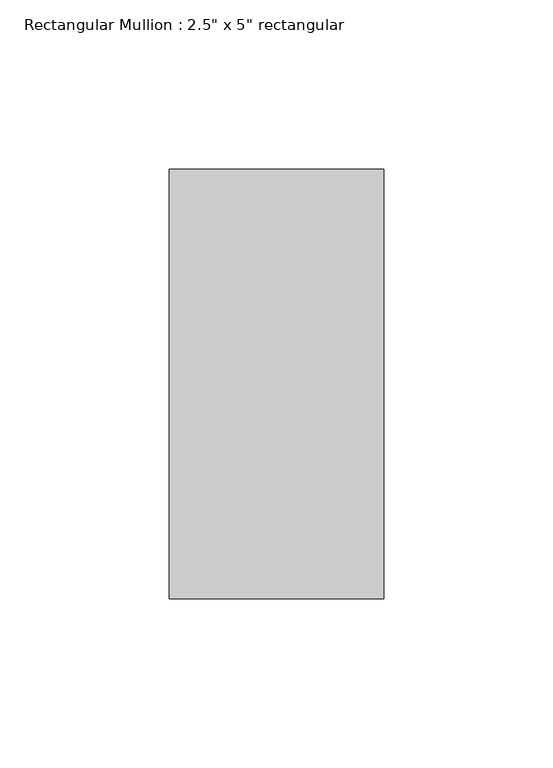
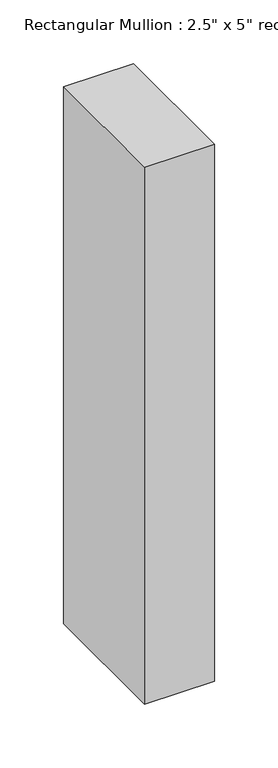
"""IFC4 building model written with IfcOpenShell, lengths in millimetres: member geometry."""

from ifc_helpers import new_model, si_unit, frame, origin, place, context, project, spatial, polyline, outline, extrude, source, transform, mapped, element, save


def member_0b7646a3(model_context):
    return source(origin(), model_context, "Body", "SweptSolid", [
        extrude(outline(polyline([(0.0, 63.5), (0.0, -63.5), (-63.5, -63.5), (-63.5, 63.5), (0.0, 63.5)])), frame((0.0, 0.0, -514.35), z_axis=(0.0, 0.0, 1.0), x_axis=(1.0, 0.0, 0.0)), (0.0, 0.0, 1.0), 514.35),
    ])


if __name__ == "__main__":
    model = new_model("IFC4")
    model_context = context("Model", 3, world=origin())
    ifc_project = project(units=[si_unit("LENGTHUNIT", "METRE", prefix="MILLI")], contexts=[model_context])
    site = spatial("IfcSite", under=ifc_project)
    building = spatial("IfcBuilding", under=site)
    placement = place(None, origin())
    member_shape = member_0b7646a3(model_context)
    element("IfcMember", 1, ObjectType="Rectangular Mullion : 2.5\" x 5\" rectangular", at=placement, inside=building, context=model_context, shape_type="MappedRepresentation", body=[
        mapped(member_shape, transform((0.0, 0.0, 0.0), x_axis=(1.0, 0.0, 0.0), y_axis=(0.0, 1.0, 0.0), z_axis=(0.0, 0.0, 1.0))),
    ])
    save(model, "model.ifc")

# Revit data of these elements
# Type "Rectangular Mullion : 2.5\" x 5\" rectangular"
#   built-in parameter 1007304 = 0.416667 (stored number, unit not read)
#   built-in parameter 1007301 = 0.104167 (stored number, unit not read)
#   built-in parameter 1007300 = 0.104167 (stored number, unit not read)
# Element 1 (IfcMember, "Rectangular Mullion : 2.5\" x 5\" rectangular")
#   Materials on its faces: "Damp-proofing"
# Materials
#   "Damp-proofing": class "Generic", colour RGB 127 127 127, transparency 0, Description = "Damp-proofing", Cost = 0
